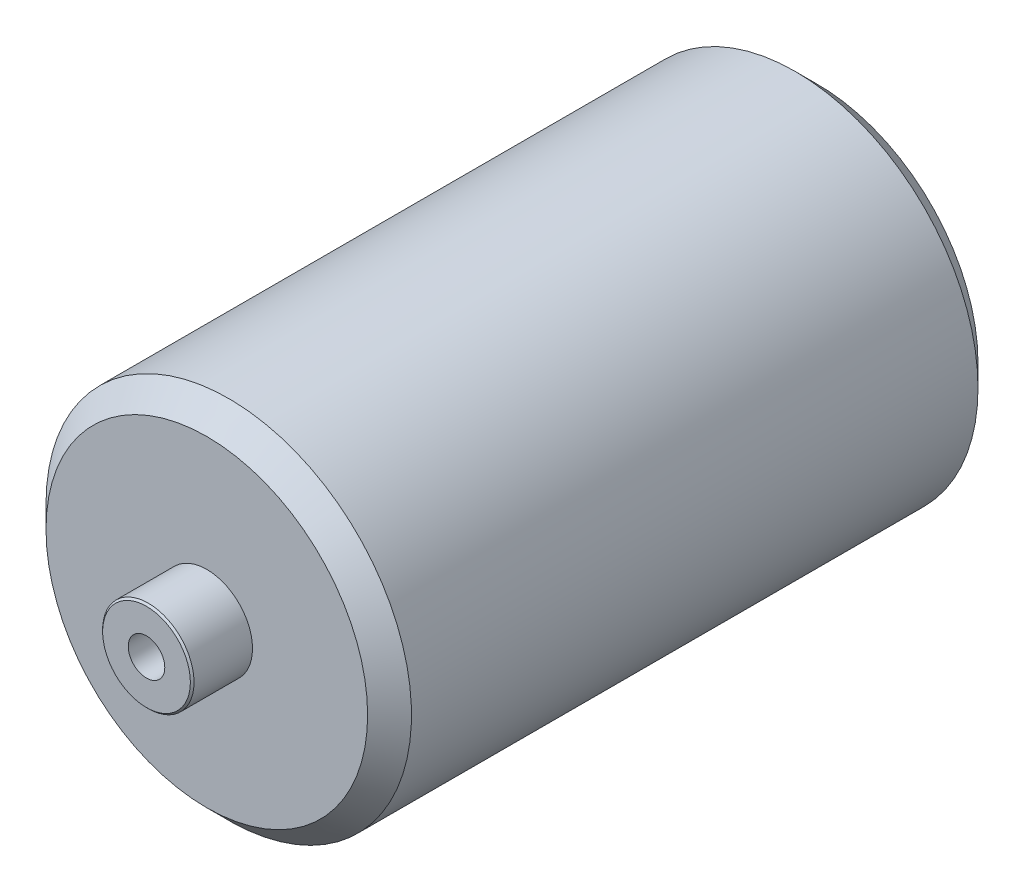
ISO-10303-21;
HEADER;
FILE_DESCRIPTION(('STEP AP214'),'2;1');
FILE_NAME('part.step','',(''),(''),'','','');
FILE_SCHEMA(('AUTOMOTIVE_DESIGN { 1 0 10303 214 1 1 1 1 }'));
ENDSEC;
DATA;
#1=APPLICATION_CONTEXT('core data for automotive mechanical design processes');
#2=APPLICATION_PROTOCOL_DEFINITION('international standard','automotive_design',2000,#1);
#3=PRODUCT_CONTEXT('',#1,'mechanical');
#4=PRODUCT('Part','Part','',(#3));
#5=PRODUCT_RELATED_PRODUCT_CATEGORY('part','',(#4));
#6=PRODUCT_DEFINITION_FORMATION('','',#4);
#7=PRODUCT_DEFINITION_CONTEXT('part definition',#1,'design');
#8=PRODUCT_DEFINITION('design','',#6,#7);
#9=PRODUCT_DEFINITION_SHAPE('','',#8);
#10=(LENGTH_UNIT() NAMED_UNIT(*) SI_UNIT(.MILLI.,.METRE.));
#11=(NAMED_UNIT(*) PLANE_ANGLE_UNIT() SI_UNIT($,.RADIAN.));
#12=(NAMED_UNIT(*) SI_UNIT($,.STERADIAN.) SOLID_ANGLE_UNIT());
#13=UNCERTAINTY_MEASURE_WITH_UNIT(LENGTH_MEASURE(1.E-05),#10,'distance_accuracy_value','');
#14=(GEOMETRIC_REPRESENTATION_CONTEXT(3) GLOBAL_UNCERTAINTY_ASSIGNED_CONTEXT((#13)) GLOBAL_UNIT_ASSIGNED_CONTEXT((#10,
#11,#12)) REPRESENTATION_CONTEXT('',''));
#15=CARTESIAN_POINT('',(0.,0.,0.));
#16=DIRECTION('',(0.,0.,1.));
#17=DIRECTION('',(1.,0.,0.));
#18=AXIS2_PLACEMENT_3D('',#15,#16,#17);
#19=CARTESIAN_POINT('',(0.,0.,167.));
#20=DIRECTION('',(0.,0.,-1.));
#21=DIRECTION('',(-1.,0.,0.));
#22=AXIS2_PLACEMENT_3D('',#19,#20,#21);
#23=CYLINDRICAL_SURFACE('',#22,50.);
#24=CARTESIAN_POINT('',(0.,0.,161.));
#25=DIRECTION('',(0.,0.,1.));
#26=DIRECTION('',(1.,0.,0.));
#27=AXIS2_PLACEMENT_3D('',#24,#25,#26);
#28=CIRCLE('',#27,50.);
#29=CARTESIAN_POINT('',(-50.,0.,161.));
#30=VERTEX_POINT('',#29);
#31=EDGE_CURVE('E49',#30,#30,#28,.F.);
#32=CARTESIAN_POINT('',(0.,0.,6.00000000000017));
#33=DIRECTION('',(0.,0.,1.));
#34=DIRECTION('',(1.,0.,0.));
#35=AXIS2_PLACEMENT_3D('',#32,#33,#34);
#36=CIRCLE('',#35,50.);
#37=CARTESIAN_POINT('',(-50.,0.,6.00000000000017));
#38=VERTEX_POINT('',#37);
#39=EDGE_CURVE('E96',#38,#38,#36,.T.);
#40=CARTESIAN_POINT('',(-50.,0.,161.));
#41=CARTESIAN_POINT('',(-50.,0.,159.385416666667));
#42=CARTESIAN_POINT('',(-50.,0.,157.770833333333));
#43=CARTESIAN_POINT('',(-50.,0.,154.541666666667));
#44=CARTESIAN_POINT('',(-50.,0.,152.927083333333));
#45=CARTESIAN_POINT('',(-50.,0.,149.697916666667));
#46=CARTESIAN_POINT('',(-50.,0.,148.083333333333));
#47=CARTESIAN_POINT('',(-50.,0.,144.854166666667));
#48=CARTESIAN_POINT('',(-50.,0.,143.239583333333));
#49=CARTESIAN_POINT('',(-50.,0.,140.010416666667));
#50=CARTESIAN_POINT('',(-50.,0.,138.395833333333));
#51=CARTESIAN_POINT('',(-50.,0.,135.166666666667));
#52=CARTESIAN_POINT('',(-50.,0.,133.552083333333));
#53=CARTESIAN_POINT('',(-50.,0.,130.322916666667));
#54=CARTESIAN_POINT('',(-50.,0.,128.708333333333));
#55=CARTESIAN_POINT('',(-50.,0.,125.479166666667));
#56=CARTESIAN_POINT('',(-50.,0.,123.864583333333));
#57=CARTESIAN_POINT('',(-50.,0.,120.635416666667));
#58=CARTESIAN_POINT('',(-50.,0.,119.020833333333));
#59=CARTESIAN_POINT('',(-50.,0.,115.791666666667));
#60=CARTESIAN_POINT('',(-50.,0.,114.177083333333));
#61=CARTESIAN_POINT('',(-50.,0.,110.947916666667));
#62=CARTESIAN_POINT('',(-50.,0.,109.333333333333));
#63=CARTESIAN_POINT('',(-50.,0.,106.104166666667));
#64=CARTESIAN_POINT('',(-50.,0.,104.489583333333));
#65=CARTESIAN_POINT('',(-50.,0.,101.260416666667));
#66=CARTESIAN_POINT('',(-50.,0.,99.6458333333335));
#67=CARTESIAN_POINT('',(-50.,0.,96.4166666666668));
#68=CARTESIAN_POINT('',(-50.,0.,94.8020833333335));
#69=CARTESIAN_POINT('',(-50.,0.,91.5729166666668));
#70=CARTESIAN_POINT('',(-50.,0.,89.9583333333335));
#71=CARTESIAN_POINT('',(-50.,0.,86.7291666666668));
#72=CARTESIAN_POINT('',(-50.,0.,85.1145833333335));
#73=CARTESIAN_POINT('',(-50.,0.,81.8854166666668));
#74=CARTESIAN_POINT('',(-50.,0.,80.2708333333335));
#75=CARTESIAN_POINT('',(-50.,0.,77.0416666666668));
#76=CARTESIAN_POINT('',(-50.,0.,75.4270833333335));
#77=CARTESIAN_POINT('',(-50.,0.,72.1979166666668));
#78=CARTESIAN_POINT('',(-50.,0.,70.5833333333335));
#79=CARTESIAN_POINT('',(-50.,0.,67.3541666666668));
#80=CARTESIAN_POINT('',(-50.,0.,65.7395833333335));
#81=CARTESIAN_POINT('',(-50.,0.,62.5104166666668));
#82=CARTESIAN_POINT('',(-50.,0.,60.8958333333335));
#83=CARTESIAN_POINT('',(-50.,0.,57.6666666666668));
#84=CARTESIAN_POINT('',(-50.,0.,56.0520833333335));
#85=CARTESIAN_POINT('',(-50.,0.,52.8229166666668));
#86=CARTESIAN_POINT('',(-50.,0.,51.2083333333335));
#87=CARTESIAN_POINT('',(-50.,0.,47.9791666666668));
#88=CARTESIAN_POINT('',(-50.,0.,46.3645833333335));
#89=CARTESIAN_POINT('',(-50.,0.,43.1354166666668));
#90=CARTESIAN_POINT('',(-50.,0.,41.5208333333335));
#91=CARTESIAN_POINT('',(-50.,0.,38.2916666666668));
#92=CARTESIAN_POINT('',(-50.,0.,36.6770833333335));
#93=CARTESIAN_POINT('',(-50.,0.,33.4479166666668));
#94=CARTESIAN_POINT('',(-50.,0.,31.8333333333335));
#95=CARTESIAN_POINT('',(-50.,0.,28.6041666666668));
#96=CARTESIAN_POINT('',(-50.,0.,26.9895833333335));
#97=CARTESIAN_POINT('',(-50.,0.,23.7604166666668));
#98=CARTESIAN_POINT('',(-50.,0.,22.1458333333335));
#99=CARTESIAN_POINT('',(-50.,0.,18.9166666666668));
#100=CARTESIAN_POINT('',(-50.,0.,17.3020833333335));
#101=CARTESIAN_POINT('',(-50.,0.,14.0729166666668));
#102=CARTESIAN_POINT('',(-50.,0.,12.4583333333335));
#103=CARTESIAN_POINT('',(-50.,0.,9.22916666666684));
#104=CARTESIAN_POINT('',(-50.,0.,7.61458333333351));
#105=CARTESIAN_POINT('',(-50.,0.,6.00000000000017));
#106=B_SPLINE_CURVE_WITH_KNOTS('',3,(#40,#41,#42,#43,#44,#45,#46,#47,#48,#49,#50,#51,#52,#53,
#54,#55,#56,#57,#58,#59,#60,#61,#62,#63,#64,#65,#66,#67,#68,#69,#70,#71,#72,#73,#74,#75,#76,#77,
#78,#79,#80,#81,#82,#83,#84,#85,#86,#87,#88,#89,#90,#91,#92,#93,#94,#95,#96,#97,#98,#99,#100,
#101,#102,#103,#104,#105),.UNSPECIFIED.,.F.,.F.,(4,2,2,2,2,2,2,2,2,2,2,2,2,2,2,2,2,2,2,2,2,2,2,
2,2,2,2,2,2,2,2,2,4),(0.,4.84374999999998,9.68749999999999,14.53125,19.375,24.21875,29.0625,
33.90625,38.75,43.59375,48.4375,53.28125,58.125,62.96875,67.8125,72.65625,77.5,82.34375,87.1875,
92.03125,96.875,101.71875,106.5625,111.40625,116.25,121.09375,125.9375,130.78125,135.625,
140.46875,145.3125,150.15625,155.),.UNSPECIFIED.);
#107=EDGE_CURVE('BSEAM41',#30,#38,#106,.T.);
#108=ORIENTED_EDGE('',*,*,#31,.T.);
#109=ORIENTED_EDGE('',*,*,#39,.T.);
#110=ORIENTED_EDGE('',*,*,#107,.T.);
#111=ORIENTED_EDGE('',*,*,#107,.F.);
#112=EDGE_LOOP('',(#108,#110,#109,#111));
#113=FACE_BOUND('',#112,.T.);
#114=ADVANCED_FACE('F41',(#113),#23,.T.);
#115=CARTESIAN_POINT('',(0.,0.,167.));
#116=DIRECTION('',(0.,0.,1.));
#117=DIRECTION('',(1.,0.,0.));
#118=AXIS2_PLACEMENT_3D('',#115,#116,#117);
#119=PLANE('',#118);
#120=CARTESIAN_POINT('',(0.,0.,167.));
#121=DIRECTION('',(0.,0.,1.));
#122=DIRECTION('',(1.,0.,0.));
#123=AXIS2_PLACEMENT_3D('',#120,#121,#122);
#124=CIRCLE('',#123,44.0000000000002);
#125=CARTESIAN_POINT('',(44.0000000000002,0.,167.));
#126=VERTEX_POINT('',#125);
#127=EDGE_CURVE('E94',#126,#126,#124,.T.);
#128=ORIENTED_EDGE('',*,*,#127,.T.);
#129=EDGE_LOOP('',(#128));
#130=FACE_BOUND('',#129,.T.);
#131=CARTESIAN_POINT('',(0.,0.,167.));
#132=DIRECTION('',(0.,0.,1.));
#133=DIRECTION('',(1.,0.,0.));
#134=AXIS2_PLACEMENT_3D('',#131,#132,#133);
#135=CIRCLE('',#134,12.5);
#136=CARTESIAN_POINT('',(12.5,0.,167.));
#137=VERTEX_POINT('',#136);
#138=EDGE_CURVE('E80',#137,#137,#135,.T.);
#139=ORIENTED_EDGE('',*,*,#138,.F.);
#140=EDGE_LOOP('',(#139));
#141=FACE_BOUND('',#140,.T.);
#142=ADVANCED_FACE('F111',(#130,#141),#119,.T.);
#143=CARTESIAN_POINT('',(0.,0.,0.));
#144=DIRECTION('',(0.,0.,1.));
#145=DIRECTION('',(1.,0.,0.));
#146=AXIS2_PLACEMENT_3D('',#143,#144,#145);
#147=PLANE('',#146);
#148=CARTESIAN_POINT('',(0.,0.,0.));
#149=DIRECTION('',(0.,0.,1.));
#150=DIRECTION('',(1.,0.,0.));
#151=AXIS2_PLACEMENT_3D('',#148,#149,#150);
#152=CIRCLE('',#151,43.9999999999999);
#153=CARTESIAN_POINT('',(43.9999999999999,0.,0.));
#154=VERTEX_POINT('',#153);
#155=EDGE_CURVE('E11',#154,#154,#152,.F.);
#156=ORIENTED_EDGE('',*,*,#155,.T.);
#157=EDGE_LOOP('',(#156));
#158=FACE_BOUND('',#157,.T.);
#159=CARTESIAN_POINT('',(0.,0.,0.));
#160=DIRECTION('',(0.,0.,-1.));
#161=DIRECTION('',(-1.,0.,0.));
#162=AXIS2_PLACEMENT_3D('',#159,#160,#161);
#163=CIRCLE('',#162,12.5);
#164=CARTESIAN_POINT('',(-12.5,0.,0.));
#165=VERTEX_POINT('',#164);
#166=EDGE_CURVE('E76',#165,#165,#163,.T.);
#167=ORIENTED_EDGE('',*,*,#166,.F.);
#168=EDGE_LOOP('',(#167));
#169=FACE_BOUND('',#168,.T.);
#170=ADVANCED_FACE('F112',(#158,#169),#147,.F.);
#171=CARTESIAN_POINT('',(0.,0.,183.5));
#172=DIRECTION('',(0.,0.,-1.));
#173=DIRECTION('',(-1.,0.,0.));
#174=AXIS2_PLACEMENT_3D('',#171,#172,#173);
#175=CYLINDRICAL_SURFACE('',#174,12.5);
#176=CARTESIAN_POINT('',(0.,0.,183.));
#177=DIRECTION('',(0.,0.,1.));
#178=DIRECTION('',(1.,0.,0.));
#179=AXIS2_PLACEMENT_3D('',#176,#177,#178);
#180=CIRCLE('',#179,12.5);
#181=CARTESIAN_POINT('',(12.5,0.,183.));
#182=VERTEX_POINT('',#181);
#183=EDGE_CURVE('E95',#182,#182,#180,.F.);
#184=ORIENTED_EDGE('',*,*,#183,.T.);
#185=EDGE_LOOP('',(#184));
#186=FACE_BOUND('',#185,.T.);
#187=ORIENTED_EDGE('',*,*,#138,.T.);
#188=EDGE_LOOP('',(#187));
#189=FACE_BOUND('',#188,.T.);
#190=ADVANCED_FACE('F117',(#186,#189),#175,.T.);
#191=CARTESIAN_POINT('',(0.,0.,183.5));
#192=DIRECTION('',(0.,0.,1.));
#193=DIRECTION('',(1.,0.,0.));
#194=AXIS2_PLACEMENT_3D('',#191,#192,#193);
#195=PLANE('',#194);
#196=CARTESIAN_POINT('',(0.,0.,183.5));
#197=DIRECTION('',(0.,0.,1.));
#198=DIRECTION('',(1.,0.,0.));
#199=AXIS2_PLACEMENT_3D('',#196,#197,#198);
#200=CIRCLE('',#199,12.);
#201=CARTESIAN_POINT('',(12.,0.,183.5));
#202=VERTEX_POINT('',#201);
#203=EDGE_CURVE('E86',#202,#202,#200,.T.);
#204=ORIENTED_EDGE('',*,*,#203,.T.);
#205=EDGE_LOOP('',(#204));
#206=FACE_BOUND('',#205,.T.);
#207=CARTESIAN_POINT('',(0.,0.,183.5));
#208=DIRECTION('',(0.,0.,1.));
#209=DIRECTION('',(1.,0.,0.));
#210=AXIS2_PLACEMENT_3D('',#207,#208,#209);
#211=CIRCLE('',#210,4.99999999999999);
#212=CARTESIAN_POINT('',(4.99999999999999,0.,183.5));
#213=VERTEX_POINT('',#212);
#214=EDGE_CURVE('E70',#213,#213,#211,.T.);
#215=ORIENTED_EDGE('',*,*,#214,.F.);
#216=EDGE_LOOP('',(#215));
#217=FACE_BOUND('',#216,.T.);
#218=ADVANCED_FACE('F119',(#206,#217),#195,.T.);
#219=CARTESIAN_POINT('',(0.,0.,-16.5));
#220=DIRECTION('',(0.,0.,1.));
#221=DIRECTION('',(1.,0.,0.));
#222=AXIS2_PLACEMENT_3D('',#219,#220,#221);
#223=CYLINDRICAL_SURFACE('',#222,12.5);
#224=CARTESIAN_POINT('',(0.,0.,-16.));
#225=DIRECTION('',(0.,0.,-1.));
#226=DIRECTION('',(-1.,0.,0.));
#227=AXIS2_PLACEMENT_3D('',#224,#225,#226);
#228=CIRCLE('',#227,12.5);
#229=CARTESIAN_POINT('',(-12.5,0.,-16.));
#230=VERTEX_POINT('',#229);
#231=EDGE_CURVE('E87',#230,#230,#228,.F.);
#232=ORIENTED_EDGE('',*,*,#231,.T.);
#233=EDGE_LOOP('',(#232));
#234=FACE_BOUND('',#233,.T.);
#235=ORIENTED_EDGE('',*,*,#166,.T.);
#236=EDGE_LOOP('',(#235));
#237=FACE_BOUND('',#236,.T.);
#238=ADVANCED_FACE('F130',(#234,#237),#223,.T.);
#239=CARTESIAN_POINT('',(0.,0.,-16.5));
#240=DIRECTION('',(0.,0.,-1.));
#241=DIRECTION('',(-1.,0.,0.));
#242=AXIS2_PLACEMENT_3D('',#239,#240,#241);
#243=PLANE('',#242);
#244=CARTESIAN_POINT('',(0.,0.,-16.5));
#245=DIRECTION('',(0.,0.,-1.));
#246=DIRECTION('',(-1.,0.,0.));
#247=AXIS2_PLACEMENT_3D('',#244,#245,#246);
#248=CIRCLE('',#247,12.);
#249=CARTESIAN_POINT('',(-12.,0.,-16.5));
#250=VERTEX_POINT('',#249);
#251=EDGE_CURVE('E82',#250,#250,#248,.T.);
#252=ORIENTED_EDGE('',*,*,#251,.T.);
#253=EDGE_LOOP('',(#252));
#254=FACE_BOUND('',#253,.T.);
#255=CARTESIAN_POINT('',(0.,0.,-16.5));
#256=DIRECTION('',(0.,0.,-1.));
#257=DIRECTION('',(-1.,0.,0.));
#258=AXIS2_PLACEMENT_3D('',#255,#256,#257);
#259=CIRCLE('',#258,5.);
#260=CARTESIAN_POINT('',(-5.,0.,-16.5));
#261=VERTEX_POINT('',#260);
#262=EDGE_CURVE('E67',#261,#261,#259,.T.);
#263=ORIENTED_EDGE('',*,*,#262,.F.);
#264=EDGE_LOOP('',(#263));
#265=FACE_BOUND('',#264,.T.);
#266=ADVANCED_FACE('F173',(#254,#265),#243,.T.);
#267=CARTESIAN_POINT('',(0.,0.,42.5));
#268=DIRECTION('',(0.,0.,-1.));
#269=DIRECTION('',(-1.,0.,0.));
#270=AXIS2_PLACEMENT_3D('',#267,#268,#269);
#271=CONICAL_SURFACE('',#270,4.99999999999999,1.02974425867665);
#272=CARTESIAN_POINT('',(0.,0.,45.5043030951378));
#273=VERTEX_POINT('',#272);
#274=VERTEX_LOOP('',#273);
#275=FACE_BOUND('',#274,.T.);
#276=CARTESIAN_POINT('',(0.,0.,42.5));
#277=DIRECTION('',(0.,0.,-1.));
#278=DIRECTION('',(-1.,0.,0.));
#279=AXIS2_PLACEMENT_3D('',#276,#277,#278);
#280=CIRCLE('',#279,4.99999999999999);
#281=CARTESIAN_POINT('',(-4.99999999999999,0.,42.5));
#282=VERTEX_POINT('',#281);
#283=EDGE_CURVE('E68',#282,#282,#280,.T.);
#284=ORIENTED_EDGE('',*,*,#283,.T.);
#285=EDGE_LOOP('',(#284));
#286=FACE_BOUND('',#285,.T.);
#287=ADVANCED_FACE('F169',(#275,#286),#271,.F.);
#288=CARTESIAN_POINT('',(0.,0.,-16.5));
#289=DIRECTION('',(0.,0.,-1.));
#290=DIRECTION('',(-1.,0.,0.));
#291=AXIS2_PLACEMENT_3D('',#288,#289,#290);
#292=CYLINDRICAL_SURFACE('',#291,5.);
#293=ORIENTED_EDGE('',*,*,#283,.F.);
#294=EDGE_LOOP('',(#293));
#295=FACE_BOUND('',#294,.T.);
#296=ORIENTED_EDGE('',*,*,#262,.T.);
#297=EDGE_LOOP('',(#296));
#298=FACE_BOUND('',#297,.T.);
#299=ADVANCED_FACE('F58',(#295,#298),#292,.F.);
#300=CARTESIAN_POINT('',(0.,0.,124.5));
#301=DIRECTION('',(0.,0.,1.));
#302=DIRECTION('',(1.,0.,0.));
#303=AXIS2_PLACEMENT_3D('',#300,#301,#302);
#304=CONICAL_SURFACE('',#303,4.99999999999998,1.02974425867665);
#305=CARTESIAN_POINT('',(0.,0.,121.495696904862));
#306=VERTEX_POINT('',#305);
#307=VERTEX_LOOP('',#306);
#308=FACE_BOUND('',#307,.T.);
#309=CARTESIAN_POINT('',(0.,0.,124.5));
#310=DIRECTION('',(0.,0.,1.));
#311=DIRECTION('',(1.,0.,0.));
#312=AXIS2_PLACEMENT_3D('',#309,#310,#311);
#313=CIRCLE('',#312,4.99999999999998);
#314=CARTESIAN_POINT('',(4.99999999999998,0.,124.5));
#315=VERTEX_POINT('',#314);
#316=EDGE_CURVE('E61',#315,#315,#313,.T.);
#317=ORIENTED_EDGE('',*,*,#316,.T.);
#318=EDGE_LOOP('',(#317));
#319=FACE_BOUND('',#318,.T.);
#320=ADVANCED_FACE('F57',(#308,#319),#304,.F.);
#321=CARTESIAN_POINT('',(0.,0.,183.5));
#322=DIRECTION('',(0.,0.,1.));
#323=DIRECTION('',(1.,0.,0.));
#324=AXIS2_PLACEMENT_3D('',#321,#322,#323);
#325=CYLINDRICAL_SURFACE('',#324,4.99999999999998);
#326=ORIENTED_EDGE('',*,*,#316,.F.);
#327=EDGE_LOOP('',(#326));
#328=FACE_BOUND('',#327,.T.);
#329=ORIENTED_EDGE('',*,*,#214,.T.);
#330=EDGE_LOOP('',(#329));
#331=FACE_BOUND('',#330,.T.);
#332=ADVANCED_FACE('F56',(#328,#331),#325,.F.);
#333=CARTESIAN_POINT('',(0.,0.,-16.5));
#334=DIRECTION('',(0.,0.,1.));
#335=DIRECTION('',(1.,0.,0.));
#336=AXIS2_PLACEMENT_3D('',#333,#334,#335);
#337=CONICAL_SURFACE('',#336,12.,0.785398163397459);
#338=ORIENTED_EDGE('',*,*,#231,.F.);
#339=EDGE_LOOP('',(#338));
#340=FACE_BOUND('',#339,.T.);
#341=ORIENTED_EDGE('',*,*,#251,.F.);
#342=EDGE_LOOP('',(#341));
#343=FACE_BOUND('',#342,.T.);
#344=ADVANCED_FACE('F139',(#340,#343),#337,.T.);
#345=CARTESIAN_POINT('',(0.,0.,183.5));
#346=DIRECTION('',(0.,0.,-1.));
#347=DIRECTION('',(-1.,0.,0.));
#348=AXIS2_PLACEMENT_3D('',#345,#346,#347);
#349=CONICAL_SURFACE('',#348,12.,0.785398163397466);
#350=ORIENTED_EDGE('',*,*,#183,.F.);
#351=EDGE_LOOP('',(#350));
#352=FACE_BOUND('',#351,.T.);
#353=ORIENTED_EDGE('',*,*,#203,.F.);
#354=EDGE_LOOP('',(#353));
#355=FACE_BOUND('',#354,.T.);
#356=ADVANCED_FACE('F108',(#352,#355),#349,.T.);
#357=CARTESIAN_POINT('',(0.,0.,167.));
#358=DIRECTION('',(0.,0.,-1.));
#359=DIRECTION('',(-1.,0.,0.));
#360=AXIS2_PLACEMENT_3D('',#357,#358,#359);
#361=CONICAL_SURFACE('',#360,44.0000000000002,0.785398163397447);
#362=ORIENTED_EDGE('',*,*,#31,.F.);
#363=EDGE_LOOP('',(#362));
#364=FACE_BOUND('',#363,.T.);
#365=ORIENTED_EDGE('',*,*,#127,.F.);
#366=EDGE_LOOP('',(#365));
#367=FACE_BOUND('',#366,.T.);
#368=ADVANCED_FACE('F102',(#364,#367),#361,.T.);
#369=CARTESIAN_POINT('',(0.,0.,6.00000000000014));
#370=DIRECTION('',(0.,0.,1.));
#371=DIRECTION('',(1.,0.,0.));
#372=AXIS2_PLACEMENT_3D('',#369,#370,#371);
#373=CONICAL_SURFACE('',#372,50.,0.785398163397449);
#374=ORIENTED_EDGE('',*,*,#155,.F.);
#375=EDGE_LOOP('',(#374));
#376=FACE_BOUND('',#375,.T.);
#377=ORIENTED_EDGE('',*,*,#39,.F.);
#378=EDGE_LOOP('',(#377));
#379=FACE_BOUND('',#378,.T.);
#380=ADVANCED_FACE('F42',(#376,#379),#373,.T.);
#381=CLOSED_SHELL('',(#114,#142,#170,#190,#218,#238,#266,#287,#299,#320,#332,#344,#356,#368,#380));
#382=MANIFOLD_SOLID_BREP('B2',#381);
#383=ADVANCED_BREP_SHAPE_REPRESENTATION('',(#18,#382),#14);
#384=SHAPE_DEFINITION_REPRESENTATION(#9,#383);
ENDSEC;
END-ISO-10303-21;
